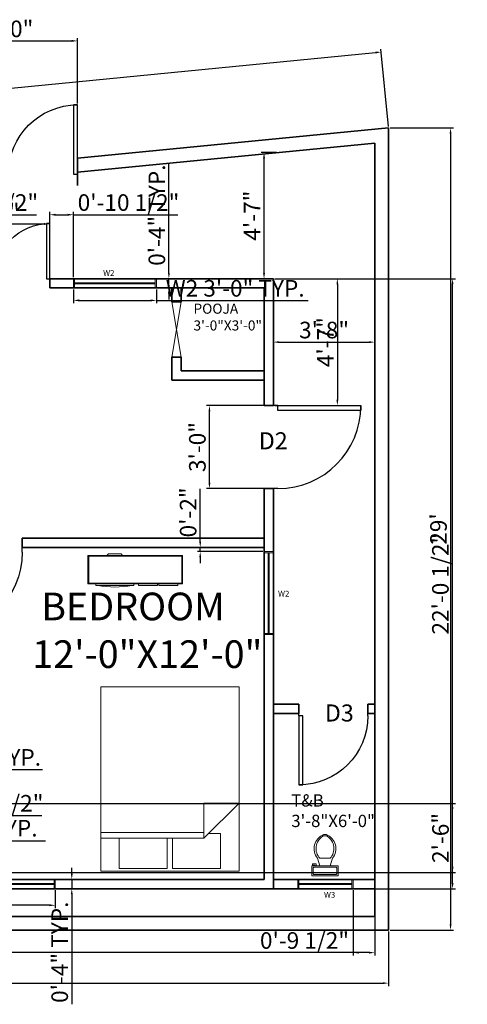
# Model space of a CAD drawing. Units: inches. Extents: x 2165 to 6441, y 2023 to 4425.
# Tile 3 of 4: x 2534 to 2728, y 2025 to 2452. Entities that reach past the tile are written whole.
import ezdxf

# ---------------------------------------------------------------- set-up
doc = ezdxf.new("R2010")
doc.units = ezdxf.units.IN
for name, color, linetype, lineweight in [('A-ANNO-DIMS', 7, 'Continuous', 18), ('A-ANNO-TEXT', 1, 'Continuous', 18), ('A-AREA-IDEN', 1, 'Continuous', 25), ('A-FLOR-FIXT', 9, 'Continuous', 18), ('C-PROP', 7, 'Continuous', 35), ('doors', 5, 'Continuous', 25), ('furniture', 9, 'Continuous', 18), ('walls', 7, 'Continuous', 35), ('windows', 72, 'Continuous', 18)]:
    doc.layers.add(name, color=color, linetype=linetype, lineweight=lineweight)
doc.styles.get("Standard").update_dxf_attribs({"font": 'arial.ttf'})
doc.dimstyles.new('ISO-25', dxfattribs={"dimtxt": 7.203125, "dimasz": 2.5, "dimexe": 1.25, "dimexo": 0.625, "dimtad": 1, "dimdec": 0, "dimlunit": 4, "dimtxsty": 'Standard', "dimcen": 2.5, "dimadec": 0, "dimazin": 0, "dimtfac": 1, "dimtdec": 0, "dimtmove": 0, "dimatfit": 3, "dimfxl": 1, "dimarcsym": 0})

# ---------------------------------------------------------------- blocks, each defined once
blk = doc.blocks.new('*U2')
for p, q in [((0, 0), (0, -5)), ((30, 0), (30, -5))]:
    blk.add_line(p, q)
blk.add_lwpolyline([(0, 0), (0, 30), (1.75, 30), (1.75, 0)], close=True)
blk.add_arc((0, 0), 30, 0, 90)
blk = doc.blocks.new('Bed - Queen')
for p, q in [((0, -80.00003), (0, 0)), ((0, 0), (59.99999, 0)), ((59.99999, 0), (59.99999, -80.00003)), ((7.99999, -1.2), (28.79998, -1.2)), ((7.99999, -14.4), (7.99999, -1.2)), ((28.79998, -1.2), (28.79998, -14.4)), ((31.19999, -1.2), (51.99999, -1.2)), ((31.19999, -14.4), (31.19999, -1.2)), ((51.99999, -1.2), (51.99999, -16.4)), ((0, -14.4), (44.8, -14.4)), ((44.8, -16.8), (0, -16.8)), ((59.99999, -29.6), (44.8, -14.4)), ((44.8, -14.4), (44.8, -29.6)), ((51.99999, -16.4), (46.79936, -16.4)), ((44.8, -29.6), (59.99999, -29.6)), ((59.99999, -80.00003), (0, -80.00003))]:
    blk.add_line(p, q)
blk = doc.blocks.new('Toilet - top')
for p, q in [((9.5, -6), (9.5, -2)), ((-10, -8.5), (-8, -8.5)), ((-10, -9.5), (-10, -8.5)), ((-7, -9.5), (-10, -9.5)), ((-8, -8.5), (-8, -8)), ((-7, -8), (-7, -9.5)), ((-4, -8), (-6, -14)), ((4, -14), (-4, -14)), ((4, -8), (6, -14))]:
    blk.add_line(p, q)
blk.add_lwpolyline([(10.5, -8), (10.5, 0), (-10.5, 0), (-10.5, -8)], close=True)
for points in [[(-9.5, -2), (-9.5, -6)], [(8.5, -1), (-8.5, -1)], [(-8.5, -7), (8.5, -7)]]:
    blk.add_lwpolyline(points)
for centre, radius, start, end in [((-8.62, -1.88), 0.884, 81.8699, 188.1301), ((-8.62, -6.12), 0.884, 171.8699, 278.1301), ((8.62, -1.88), 0.884, 351.8699, 98.1301), ((8.62, -6.12), 0.884, 261.8699, 8.1301), ((3.52, -21.58), 12.17, 141.46911, 247.97143), ((4.2, -21.82), 11.33, 136.36773, 238.94682), ((-3.52, -21.58), 12.17, 292.02843, 38.53071), ((-4.2, -21.82), 11.33, 301.05301, 43.63209), ((0, -27.88), 4, 245.73182, 294.26817), ((0, -29), 4, 254.86053, 285.13947)]:
    blk.add_arc(centre, radius, start, end)
blk = doc.blocks.new('*D8')
at = {"layer": 'A-ANNO-DIMS', "color": 0, "lineweight": -2, "transparency": 16777216}
for p, q in [((2693.62, 2405.41), (2690.35, 2438.92)), ((2200.96, 2389.92), (2687.99, 2437.43)), ((2201.62, 2357.41), (2198.35, 2390.92))]:
    blk.add_line(p, q, dxfattribs=at)
at = {"layer": 'A-ANNO-DIMS', "color": 0, "transparency": 16777216}
for points in [[(2687.95, 2437.85), (2688.03, 2437.02), (2690.48, 2437.67)], [(2200.92, 2390.33), (2201, 2389.5), (2198.48, 2389.67)]]:
    blk.add_solid(points, dxfattribs=at)
at = {"layer": 'Defpoints', "color": 0, "transparency": 16777216}
for p in [(2690.48, 2437.67), (2693.68, 2404.78), (2201.68, 2356.78)]:
    blk.add_point(p, dxfattribs=at)
at = {"layer": 'A-ANNO-DIMS', "color": 0, "transparency": 16777216, "insert": (2444.06, 2417.9), "char_height": 7.203, "attachment_point": 5, "rotation": 5.5722}
blk.add_mtext('41\'-2"', dxfattribs=at)
blk = doc.blocks.new('*D9')
at = {"layer": 'A-ANNO-DIMS', "color": 0, "lineweight": -2, "transparency": 16777216}
for p, q in [((2694.31, 2404.78), (2721.8, 2404.78)), ((2720.55, 2402.28), (2720.55, 2059.28)), ((2694.31, 2056.78), (2721.8, 2056.78))]:
    blk.add_line(p, q, dxfattribs=at)
at = {"layer": 'A-ANNO-DIMS', "color": 0, "transparency": 16777216}
for points in [[(2720.14, 2402.28), (2720.97, 2402.28), (2720.55, 2404.78)], [(2720.14, 2059.28), (2720.97, 2059.28), (2720.55, 2056.78)]]:
    blk.add_solid(points, dxfattribs=at)
at = {"layer": 'Defpoints', "color": 0, "transparency": 16777216}
for p in [(2693.68, 2404.78), (2693.68, 2056.78), (2720.55, 2056.78)]:
    blk.add_point(p, dxfattribs=at)
at = {"layer": 'A-ANNO-DIMS', "color": 0, "transparency": 16777216, "insert": (2716.25, 2230.78), "char_height": 7.203, "attachment_point": 5, "rotation": 90}
blk.add_mtext("29'", dxfattribs=at)
blk = doc.blocks.new('*D11')
at = {"layer": 'A-ANNO-DIMS', "color": 0, "lineweight": -2, "transparency": 16777216}
for p, q in [((2201.68, 2056.16), (2201.68, 2032.56)), ((2693.68, 2056.16), (2693.68, 2032.56)), ((2204.18, 2033.81), (2691.18, 2033.81))]:
    blk.add_line(p, q, dxfattribs=at)
at = {"layer": 'A-ANNO-DIMS', "color": 0, "transparency": 16777216}
for points in [[(2204.18, 2034.23), (2204.18, 2033.39), (2201.68, 2033.81)], [(2691.18, 2034.23), (2691.18, 2033.39), (2693.68, 2033.81)]]:
    blk.add_solid(points, dxfattribs=at)
at = {"layer": 'Defpoints', "color": 0, "transparency": 16777216}
for p in [(2201.68, 2056.78), (2693.68, 2056.78), (2693.68, 2033.81)]:
    blk.add_point(p, dxfattribs=at)
at = {"layer": 'A-ANNO-DIMS', "color": 0, "transparency": 16777216, "insert": (2447.68, 2038.05), "char_height": 7.203, "attachment_point": 5}
blk.add_mtext("41'", dxfattribs=at)
blk = doc.blocks.new('*D17')
at = {"layer": 'A-ANNO-DIMS', "color": 0, "lineweight": -2, "transparency": 16777216}
for p, q in [((2643.68, 2312.47), (2643.68, 2313.09)), ((2646.18, 2311.84), (2685.18, 2311.84)), ((2687.68, 2312.47), (2687.68, 2313.09))]:
    blk.add_line(p, q, dxfattribs=at)
at = {"layer": 'A-ANNO-DIMS', "color": 0, "transparency": 16777216}
for points in [[(2646.18, 2312.26), (2646.18, 2311.42), (2643.68, 2311.84)], [(2685.18, 2312.26), (2685.18, 2311.42), (2687.68, 2311.84)]]:
    blk.add_solid(points, dxfattribs=at)
at = {"layer": 'Defpoints', "color": 0, "transparency": 16777216}
for p in [(2643.68, 2311.84), (2687.68, 2311.84), (2687.68, 2311.84)]:
    blk.add_point(p, dxfattribs=at)
at = {"layer": 'A-ANNO-DIMS', "color": 0, "transparency": 16777216, "insert": (2665.68, 2316.15), "char_height": 7.203, "attachment_point": 5}
blk.add_mtext('3\'-8"', dxfattribs=at)
blk = doc.blocks.new('Entertainment Center')
for p, q in [((-4, 0), (-5, -1)), ((4, 0), (-4, 0)), ((5, -1), (4, 0)), ((-17, -19), (-17, -1)), ((-17, -1), (43, -1)), ((-16.5, -18.5), (-16.5, -1.5)), ((-16.5, -1.5), (42.5, -1.5)), ((42.5, -1.5), (42.5, -18.5)), ((43, -1), (43, -19)), ((42.5, -18.5), (-16.5, -18.5)), ((43, -19), (-17, -19)), ((-12, -20), (-12, -19)), ((12, -20), (-12, -20)), ((12, -19), (12, -20)), ((15, -20), (15, -19)), ((27, -20), (15, -20)), ((27, -19), (27, -20)), ((28, -20), (28, -19)), ((40, -20), (28, -20)), ((40, -19), (40, -20))]:
    blk.add_line(p, q)
blk.add_arc((0, 40), 61, 259.6111, 280.3889)
blk = doc.blocks.new('*D21')
at = {"layer": 'A-ANNO-DIMS', "color": 0, "lineweight": -2, "transparency": 16777216}
for p, q in [((2645.05, 2394.07), (2638.37, 2394.07)), ((2639.62, 2341.84), (2639.62, 2391.57)), ((2643.06, 2339.34), (2638.37, 2339.34))]:
    blk.add_line(p, q, dxfattribs=at)
at = {"layer": 'A-ANNO-DIMS', "color": 0, "transparency": 16777216}
for points in [[(2639.2, 2391.57), (2640.03, 2391.57), (2639.62, 2394.07)], [(2639.2, 2341.84), (2640.03, 2341.84), (2639.62, 2339.34)]]:
    blk.add_solid(points, dxfattribs=at)
at = {"layer": 'Defpoints', "color": 0, "transparency": 16777216}
for p in [(2639.62, 2394.07), (2645.67, 2394.07), (2643.68, 2339.34)]:
    blk.add_point(p, dxfattribs=at)
at = {"layer": 'A-ANNO-DIMS', "color": 0, "transparency": 16777216, "insert": (2635.39, 2366.71), "char_height": 7.203, "attachment_point": 5, "rotation": 90}
blk.add_mtext('4\'-7"', dxfattribs=at)
blk = doc.blocks.new('WIN-W2-36IN')
for p, q in [((0, 4), (36, 4)), ((0, 0), (0, 4)), ((36, 0), (0, 0)), ((0.5, 0), (0.5, 4)), ((0.5, 2.2), (35.5, 2.2)), ((0.5, 1.8), (35.5, 1.8)), ((0.5, 1.8), (35.5, 1.8)), ((35.5, 4), (35.5, 0)), ((36, 4), (36, 0))]:
    blk.add_line(p, q)
blk = doc.blocks.new('WIN-W1-48IN')
for p, q in [((0, 4), (48, 4)), ((0, 0), (0, 4)), ((48, 0), (0, 0)), ((0.5, 0), (0.5, 4)), ((0.5, 2.2), (47.5, 2.2)), ((0.5, 1.8), (47.5, 1.8)), ((47.5, 4), (47.5, 0)), ((48, 4), (48, 0))]:
    blk.add_line(p, q)
blk = doc.blocks.new('WIN-W3-24IN')
for p, q in [((0, 4), (24, 4)), ((0, 0), (0, 4)), ((24, 0), (0, 0)), ((0.5, 0), (0.5, 4)), ((23.5, 2.2), (0.5, 2.2)), ((23.5, 1.8), (0.5, 1.8)), ((23.5, 0), (23.5, 4)), ((24, 0), (24, 4))]:
    blk.add_line(p, q)
blk = doc.blocks.new('*D26')
at = {"layer": 'A-ANNO-DIMS', "color": 0, "lineweight": -2, "transparency": 16777216}
for p, q in [((2500.99, 2074.16), (2500.99, 2066.33)), ((2549, 2074.16), (2549, 2066.33)), ((2500.99, 2067.58), (2435.15, 2067.58)), ((2546.5, 2067.58), (2503.49, 2067.58))]:
    blk.add_line(p, q, dxfattribs=at)
at = {"layer": 'A-ANNO-DIMS', "color": 0, "transparency": 16777216}
for points in [[(2503.49, 2068), (2503.49, 2067.17), (2500.99, 2067.58)], [(2546.5, 2068), (2546.5, 2067.17), (2549, 2067.58)]]:
    blk.add_solid(points, dxfattribs=at)
at = {"layer": 'Defpoints', "color": 0, "transparency": 16777216}
for p in [(2500.99, 2074.78), (2549, 2074.78), (2500.99, 2067.58)]:
    blk.add_point(p, dxfattribs=at)
at = {"layer": 'A-ANNO-DIMS', "color": 0, "transparency": 16777216, "insert": (2466.82, 2071.89), "char_height": 7.2031, "attachment_point": 5}
blk.add_mtext('W1 4\'-0" TYP.', dxfattribs=at)
blk = doc.blocks.new('*D27')
at = {"layer": 'A-ANNO-DIMS', "color": 0, "lineweight": -2, "transparency": 16777216}
for p, q in [((2556.2, 2081.28), (2556.2, 2083.78)), ((2549.62, 2078.78), (2557.45, 2078.78)), ((2556.2, 2078.78), (2556.2, 2074.78)), ((2549.62, 2074.78), (2557.45, 2074.78)), ((2556.2, 2072.28), (2556.2, 2024.63))]:
    blk.add_line(p, q, dxfattribs=at)
at = {"layer": 'A-ANNO-DIMS', "color": 0, "transparency": 16777216}
for points in [[(2555.78, 2081.28), (2556.61, 2081.28), (2556.2, 2078.78)], [(2555.78, 2072.28), (2556.61, 2072.28), (2556.2, 2074.78)]]:
    blk.add_solid(points, dxfattribs=at)
at = {"layer": 'Defpoints', "color": 0, "transparency": 16777216}
for p in [(2549, 2078.78), (2549, 2074.78), (2556.2, 2074.78)]:
    blk.add_point(p, dxfattribs=at)
at = {"layer": 'A-ANNO-DIMS', "color": 0, "transparency": 16777216, "insert": (2551.89, 2047.21), "char_height": 7.203, "attachment_point": 5, "rotation": 90}
blk.add_mtext('0\'-4" TYP.', dxfattribs=at)
blk = doc.blocks.new('*D28')
at = {"layer": 'A-ANNO-DIMS', "color": 0, "lineweight": -2, "transparency": 16777216}
for p, q in [((2556.93, 2334.72), (2556.93, 2328.69)), ((2592.94, 2334.72), (2592.94, 2328.69)), ((2559.43, 2329.94), (2590.44, 2329.94)), ((2592.94, 2329.94), (2658.78, 2329.94))]:
    blk.add_line(p, q, dxfattribs=at)
at = {"layer": 'A-ANNO-DIMS', "color": 0, "transparency": 16777216}
for points in [[(2559.43, 2330.36), (2559.43, 2329.52), (2556.93, 2329.94)], [(2590.44, 2330.36), (2590.44, 2329.52), (2592.94, 2329.94)]]:
    blk.add_solid(points, dxfattribs=at)
at = {"layer": 'Defpoints', "color": 0, "transparency": 16777216}
for p in [(2556.93, 2335.34), (2592.94, 2335.34), (2592.94, 2329.94)]:
    blk.add_point(p, dxfattribs=at)
at = {"layer": 'A-ANNO-DIMS', "color": 0, "transparency": 16777216, "insert": (2627.11, 2334.25), "char_height": 7.2031, "attachment_point": 5}
blk.add_mtext('W2 3\'-0" TYP.', dxfattribs=at)
blk = doc.blocks.new('*D29')
at = {"layer": 'A-ANNO-DIMS', "color": 0, "lineweight": -2, "transparency": 16777216}
for p, q in [((2598.34, 2341.84), (2598.34, 2389.5)), ((2593.56, 2339.34), (2599.59, 2339.34)), ((2598.34, 2335.34), (2598.34, 2339.34)), ((2593.56, 2335.34), (2599.59, 2335.34)), ((2598.34, 2332.84), (2598.34, 2330.34))]:
    blk.add_line(p, q, dxfattribs=at)
at = {"layer": 'A-ANNO-DIMS', "color": 0, "transparency": 16777216}
for points in [[(2597.92, 2341.84), (2598.76, 2341.84), (2598.34, 2339.34)], [(2597.92, 2332.84), (2598.76, 2332.84), (2598.34, 2335.34)]]:
    blk.add_solid(points, dxfattribs=at)
at = {"layer": 'Defpoints', "color": 0, "transparency": 16777216}
for p in [(2592.94, 2339.34), (2598.34, 2339.34), (2592.94, 2335.34)]:
    blk.add_point(p, dxfattribs=at)
at = {"layer": 'A-ANNO-DIMS', "color": 0, "transparency": 16777216, "insert": (2594.04, 2366.92), "char_height": 7.203, "attachment_point": 5, "rotation": 90}
blk.add_mtext('0\'-4" TYP.', dxfattribs=at)
blk = doc.blocks.new('*D32')
at = {"layer": 'A-ANNO-DIMS', "color": 0, "lineweight": -2, "transparency": 16777216}
for p, q in [((2355.04, 2106.91), (2355.04, 2094.28)), ((2435.04, 2106.91), (2435.04, 2094.28)), ((2357.54, 2095.53), (2432.54, 2095.53)), ((2435.04, 2095.53), (2544.75, 2095.53))]:
    blk.add_line(p, q, dxfattribs=at)
at = {"layer": 'A-ANNO-DIMS', "color": 0, "transparency": 16777216}
for points in [[(2357.54, 2095.95), (2357.54, 2095.11), (2355.04, 2095.53)], [(2432.54, 2095.95), (2432.54, 2095.11), (2435.04, 2095.53)]]:
    blk.add_solid(points, dxfattribs=at)
at = {"layer": 'Defpoints', "color": 0, "transparency": 16777216}
for p in [(2355.04, 2107.53), (2435.04, 2107.53), (2435.04, 2095.53)]:
    blk.add_point(p, dxfattribs=at)
at = {"layer": 'A-ANNO-DIMS', "color": 0, "transparency": 16777216, "insert": (2491.14, 2100.1), "char_height": 7.2031, "attachment_point": 5}
blk.add_mtext('QUEEN BED 6\'-8" TYP.', dxfattribs=at)
blk = doc.blocks.new('*D43')
at = {"layer": 'A-ANNO-DIMS', "color": 0, "lineweight": -2, "transparency": 16777216}
for p, q in [((2461.96, 2128.52), (2461.96, 2125.2)), ((2473.4, 2128.52), (2473.4, 2125.2)), ((2464.46, 2126.45), (2470.9, 2126.45)), ((2473.4, 2126.45), (2543.44, 2126.45))]:
    blk.add_line(p, q, dxfattribs=at)
at = {"layer": 'A-ANNO-DIMS', "color": 0, "transparency": 16777216}
for points in [[(2464.46, 2126.86), (2464.46, 2126.03), (2461.96, 2126.45)], [(2470.9, 2126.86), (2470.9, 2126.03), (2473.4, 2126.45)]]:
    blk.add_solid(points, dxfattribs=at)
at = {"layer": 'Defpoints', "color": 0, "transparency": 16777216}
for p in [(2461.96, 2129.15), (2473.4, 2129.15), (2473.4, 2126.45)]:
    blk.add_point(p, dxfattribs=at)
at = {"layer": 'A-ANNO-DIMS', "color": 0, "transparency": 16777216, "insert": (2509.67, 2130.8), "char_height": 7.2031, "attachment_point": 5}
blk.add_mtext('0\'-11 1/2" TYP.', dxfattribs=at)
blk = doc.blocks.new('*D45')
at = {"layer": 'A-ANNO-DIMS', "color": 0, "lineweight": -2, "transparency": 16777216}
for p, q in [((2498.68, 2415.36), (2498.68, 2443.73)), ((2558.68, 2415.36), (2558.68, 2443.73)), ((2501.18, 2442.48), (2556.18, 2442.48))]:
    blk.add_line(p, q, dxfattribs=at)
at = {"layer": 'A-ANNO-DIMS', "color": 0, "transparency": 16777216}
for points in [[(2501.18, 2442.9), (2501.18, 2442.06), (2498.68, 2442.48)], [(2556.18, 2442.9), (2556.18, 2442.06), (2558.68, 2442.48)]]:
    blk.add_solid(points, dxfattribs=at)
at = {"layer": 'Defpoints', "color": 0, "transparency": 16777216}
for p in [(2558.68, 2442.48), (2498.68, 2414.73), (2558.68, 2414.73)]:
    blk.add_point(p, dxfattribs=at)
at = {"layer": 'A-ANNO-DIMS', "color": 0, "transparency": 16777216, "insert": (2528.68, 2446.78), "char_height": 7.203, "attachment_point": 5}
blk.add_mtext('5\'-0"', dxfattribs=at)
blk = doc.blocks.new('*D46')
at = {"layer": 'A-ANNO-DIMS', "color": 0, "lineweight": -2, "transparency": 16777216}
for p, q in [((2498.68, 2335.97), (2498.68, 2364.34)), ((2501.18, 2363.09), (2544.18, 2363.09)), ((2546.68, 2335.97), (2546.68, 2364.34))]:
    blk.add_line(p, q, dxfattribs=at)
at = {"layer": 'A-ANNO-DIMS', "color": 0, "transparency": 16777216}
for points in [[(2501.18, 2363.51), (2501.18, 2362.67), (2498.68, 2363.09)], [(2544.18, 2363.51), (2544.18, 2362.67), (2546.68, 2363.09)]]:
    blk.add_solid(points, dxfattribs=at)
at = {"layer": 'Defpoints', "color": 0, "transparency": 16777216}
for p in [(2546.68, 2363.09), (2498.68, 2335.34), (2546.68, 2335.34)]:
    blk.add_point(p, dxfattribs=at)
at = {"layer": 'A-ANNO-DIMS', "color": 0, "transparency": 16777216, "insert": (2522.68, 2367.39), "char_height": 7.203, "attachment_point": 5}
blk.add_mtext('4\'-0"', dxfattribs=at)
blk = doc.blocks.new('*D47')
at = {"layer": 'A-ANNO-DIMS', "color": 0, "lineweight": -2, "transparency": 16777216}
for p, q in [((2643.06, 2284.34), (2614.68, 2284.34)), ((2615.93, 2250.84), (2615.93, 2281.84)), ((2643.06, 2248.34), (2614.68, 2248.34))]:
    blk.add_line(p, q, dxfattribs=at)
at = {"layer": 'A-ANNO-DIMS', "color": 0, "transparency": 16777216}
for points in [[(2615.52, 2281.84), (2616.35, 2281.84), (2615.93, 2284.34)], [(2615.52, 2250.84), (2616.35, 2250.84), (2615.93, 2248.34)]]:
    blk.add_solid(points, dxfattribs=at)
at = {"layer": 'Defpoints', "color": 0, "transparency": 16777216}
for p in [(2615.93, 2284.34), (2643.68, 2284.34), (2643.68, 2248.34)]:
    blk.add_point(p, dxfattribs=at)
at = {"layer": 'A-ANNO-DIMS', "color": 0, "transparency": 16777216, "insert": (2611.63, 2266.34), "char_height": 7.203, "attachment_point": 5, "rotation": 90}
blk.add_mtext('3\'-0"', dxfattribs=at)
blk = doc.blocks.new('*D48')
at = {"layer": 'A-ANNO-DIMS', "color": 0, "lineweight": -2, "transparency": 16777216}
for p, q in [((2492.31, 2111.78), (2722.68, 2111.78)), ((2721.43, 2084.28), (2721.43, 2109.28)), ((2492.31, 2081.78), (2722.68, 2081.78))]:
    blk.add_line(p, q, dxfattribs=at)
at = {"layer": 'A-ANNO-DIMS', "color": 0, "transparency": 16777216}
for points in [[(2721.02, 2109.28), (2721.85, 2109.28), (2721.43, 2111.78)], [(2721.02, 2084.28), (2721.85, 2084.28), (2721.43, 2081.78)]]:
    blk.add_solid(points, dxfattribs=at)
at = {"layer": 'Defpoints', "color": 0, "transparency": 16777216}
for p in [(2491.68, 2111.78), (2721.43, 2111.78), (2491.68, 2081.78)]:
    blk.add_point(p, dxfattribs=at)
at = {"layer": 'A-ANNO-DIMS', "color": 0, "transparency": 16777216, "insert": (2717.13, 2096.78), "char_height": 7.203, "attachment_point": 5, "rotation": 90}
blk.add_mtext('2\'-6"', dxfattribs=at)
blk = doc.blocks.new('*D51')
at = {"layer": 'A-ANNO-DIMS', "color": 0, "lineweight": -2, "transparency": 16777216}
for p, q in [((2291.68, 2074.16), (2291.68, 2045.78)), ((2687.68, 2074.16), (2687.68, 2045.78)), ((2685.18, 2047.03), (2294.18, 2047.03))]:
    blk.add_line(p, q, dxfattribs=at)
at = {"layer": 'A-ANNO-DIMS', "color": 0, "transparency": 16777216}
for points in [[(2294.18, 2047.45), (2294.18, 2046.62), (2291.68, 2047.03)], [(2685.18, 2047.45), (2685.18, 2046.62), (2687.68, 2047.03)]]:
    blk.add_solid(points, dxfattribs=at)
at = {"layer": 'Defpoints', "color": 0, "transparency": 16777216}
for p in [(2291.68, 2074.78), (2687.68, 2074.78), (2291.68, 2047.03)]:
    blk.add_point(p, dxfattribs=at)
at = {"layer": 'A-ANNO-DIMS', "color": 0, "transparency": 16777216, "insert": (2489.68, 2051.34), "char_height": 7.203, "attachment_point": 5}
blk.add_mtext('33\'-0"', dxfattribs=at)
blk = doc.blocks.new('*D52')
at = {"layer": 'A-ANNO-DIMS', "color": 0, "lineweight": -2, "transparency": 16777216}
for p, q in [((2644.31, 2339.34), (2722.68, 2339.34)), ((2721.43, 2077.28), (2721.43, 2336.84)), ((2644.31, 2074.78), (2722.68, 2074.78))]:
    blk.add_line(p, q, dxfattribs=at)
at = {"layer": 'A-ANNO-DIMS', "color": 0, "transparency": 16777216}
for points in [[(2721.02, 2336.84), (2721.85, 2336.84), (2721.43, 2339.34)], [(2721.02, 2077.28), (2721.85, 2077.28), (2721.43, 2074.78)]]:
    blk.add_solid(points, dxfattribs=at)
at = {"layer": 'Defpoints', "color": 0, "transparency": 16777216}
for p in [(2643.68, 2339.34), (2721.43, 2339.34), (2643.68, 2074.78)]:
    blk.add_point(p, dxfattribs=at)
at = {"layer": 'A-ANNO-DIMS', "color": 0, "transparency": 16777216, "insert": (2717.08, 2207.06), "char_height": 7.203, "attachment_point": 5, "rotation": 90}
blk.add_mtext('22\'-0 1/2"', dxfattribs=at)
blk = doc.blocks.new('*D57')
at = {"layer": 'A-ANNO-DIMS', "color": 0, "lineweight": -2, "transparency": 16777216}
for p, q in [((2490.69, 2367.09), (2488.19, 2367.09)), ((2493.19, 2339.97), (2493.19, 2368.34)), ((2493.19, 2367.09), (2498.68, 2367.09)), ((2498.68, 2339.97), (2498.68, 2368.34)), ((2501.18, 2367.09), (2540.87, 2367.09))]:
    blk.add_line(p, q, dxfattribs=at)
at = {"layer": 'A-ANNO-DIMS', "color": 0, "transparency": 16777216}
for points in [[(2490.69, 2367.51), (2490.69, 2366.67), (2493.19, 2367.09)], [(2501.18, 2367.51), (2501.18, 2366.67), (2498.68, 2367.09)]]:
    blk.add_solid(points, dxfattribs=at)
at = {"layer": 'Defpoints', "color": 0, "transparency": 16777216}
for p in [(2498.68, 2367.09), (2493.19, 2339.34), (2498.68, 2339.34)]:
    blk.add_point(p, dxfattribs=at)
at = {"layer": 'A-ANNO-DIMS', "color": 0, "transparency": 16777216, "insert": (2522.28, 2371.44), "char_height": 7.203, "attachment_point": 5}
blk.add_mtext('0\'-5 1/2"', dxfattribs=at)
blk = doc.blocks.new('*D58')
at = {"layer": 'A-ANNO-DIMS', "color": 0, "lineweight": -2, "transparency": 16777216}
for p, q in [((2546.68, 2339.97), (2546.68, 2368.34)), ((2549.18, 2367.09), (2554.43, 2367.09)), ((2556.93, 2339.97), (2556.93, 2368.34)), ((2556.93, 2367.09), (2602.21, 2367.09))]:
    blk.add_line(p, q, dxfattribs=at)
at = {"layer": 'A-ANNO-DIMS', "color": 0, "transparency": 16777216}
for points in [[(2549.18, 2367.51), (2549.18, 2366.67), (2546.68, 2367.09)], [(2554.43, 2367.51), (2554.43, 2366.67), (2556.93, 2367.09)]]:
    blk.add_solid(points, dxfattribs=at)
at = {"layer": 'Defpoints', "color": 0, "transparency": 16777216}
for p in [(2556.93, 2367.09), (2546.68, 2339.34), (2556.93, 2339.34)]:
    blk.add_point(p, dxfattribs=at)
at = {"layer": 'A-ANNO-DIMS', "color": 0, "transparency": 16777216, "insert": (2580.82, 2371.44), "char_height": 7.203, "attachment_point": 5}
blk.add_mtext('0\'-10 1/2"', dxfattribs=at)
blk = doc.blocks.new('*D60')
at = {"layer": 'A-ANNO-DIMS', "color": 0, "lineweight": -2, "transparency": 16777216}
for p, q in [((2493.18, 2106.53), (2490.68, 2106.53)), ((2495.68, 2079.41), (2495.68, 2107.78)), ((2495.68, 2106.53), (2500.99, 2106.53)), ((2500.99, 2079.41), (2500.99, 2107.78)), ((2503.49, 2106.53), (2543.17, 2106.53))]:
    blk.add_line(p, q, dxfattribs=at)
at = {"layer": 'A-ANNO-DIMS', "color": 0, "transparency": 16777216}
for points in [[(2493.18, 2106.95), (2493.18, 2106.12), (2495.68, 2106.53)], [(2503.49, 2106.95), (2503.49, 2106.12), (2500.99, 2106.53)]]:
    blk.add_solid(points, dxfattribs=at)
at = {"layer": 'Defpoints', "color": 0, "transparency": 16777216}
for p in [(2500.99, 2106.53), (2495.68, 2078.78), (2500.99, 2078.78)]:
    blk.add_point(p, dxfattribs=at)
at = {"layer": 'A-ANNO-DIMS', "color": 0, "transparency": 16777216, "insert": (2524.58, 2110.88), "char_height": 7.203, "attachment_point": 5}
blk.add_mtext('0\'-5 1/2"', dxfattribs=at)
blk = doc.blocks.new('*D61')
at = {"layer": 'A-ANNO-DIMS', "color": 0, "lineweight": -2, "transparency": 16777216}
for p, q in [((2678.28, 2074.16), (2678.28, 2045.78)), ((2687.68, 2074.16), (2687.68, 2045.78)), ((2678.28, 2047.03), (2638.59, 2047.03)), ((2685.18, 2047.03), (2680.78, 2047.03))]:
    blk.add_line(p, q, dxfattribs=at)
at = {"layer": 'A-ANNO-DIMS', "color": 0, "transparency": 16777216}
for points in [[(2680.78, 2047.45), (2680.78, 2046.62), (2678.28, 2047.03)], [(2685.18, 2047.45), (2685.18, 2046.62), (2687.68, 2047.03)]]:
    blk.add_solid(points, dxfattribs=at)
at = {"layer": 'Defpoints', "color": 0, "transparency": 16777216}
for p in [(2678.28, 2074.78), (2687.68, 2074.78), (2678.28, 2047.03)]:
    blk.add_point(p, dxfattribs=at)
at = {"layer": 'A-ANNO-DIMS', "color": 0, "transparency": 16777216, "insert": (2657.18, 2051.38), "char_height": 7.203, "attachment_point": 5}
blk.add_mtext('0\'-9 1/2"', dxfattribs=at)
blk = doc.blocks.new('*D63')
at = {"layer": 'A-ANNO-DIMS', "color": 0, "lineweight": -2, "transparency": 16777216}
for p, q in [((2611.93, 2225.28), (2611.93, 2248.18)), ((2639.06, 2222.78), (2610.68, 2222.78)), ((2639.06, 2220.97), (2610.68, 2220.97)), ((2611.93, 2220.97), (2611.93, 2222.78)), ((2611.93, 2218.47), (2611.93, 2215.97))]:
    blk.add_line(p, q, dxfattribs=at)
at = {"layer": 'A-ANNO-DIMS', "color": 0, "transparency": 16777216}
for points in [[(2611.52, 2225.28), (2612.35, 2225.28), (2611.93, 2222.78)], [(2611.52, 2218.47), (2612.35, 2218.47), (2611.93, 2220.97)]]:
    blk.add_solid(points, dxfattribs=at)
at = {"layer": 'Defpoints', "color": 0, "transparency": 16777216}
for p in [(2611.93, 2222.78), (2639.68, 2222.78), (2639.68, 2220.97)]:
    blk.add_point(p, dxfattribs=at)
at = {"layer": 'A-ANNO-DIMS', "color": 0, "transparency": 16777216, "insert": (2607.63, 2237.98), "char_height": 7.203, "attachment_point": 5, "rotation": 90}
blk.add_mtext('0\'-2"', dxfattribs=at)
blk = doc.blocks.new('*D64')
at = {"layer": 'A-ANNO-DIMS', "color": 0, "lineweight": -2, "transparency": 16777216}
for p, q in [((2644.31, 2339.34), (2672.68, 2339.34)), ((2671.43, 2336.84), (2671.43, 2286.84)), ((2644.31, 2284.34), (2672.68, 2284.34))]:
    blk.add_line(p, q, dxfattribs=at)
at = {"layer": 'A-ANNO-DIMS', "color": 0, "transparency": 16777216}
for points in [[(2671.02, 2336.84), (2671.85, 2336.84), (2671.43, 2339.34)], [(2671.02, 2286.84), (2671.85, 2286.84), (2671.43, 2284.34)]]:
    blk.add_solid(points, dxfattribs=at)
at = {"layer": 'Defpoints', "color": 0, "transparency": 16777216}
for p in [(2643.68, 2339.34), (2643.68, 2284.34), (2671.43, 2284.34)]:
    blk.add_point(p, dxfattribs=at)
at = {"layer": 'A-ANNO-DIMS', "color": 0, "transparency": 16777216, "insert": (2667.21, 2311.84), "char_height": 7.203, "attachment_point": 5, "rotation": 90}
blk.add_mtext('4\'-7"', dxfattribs=at)

msp = doc.modelspace()

# ---------------------------------------------------------------- linework, layer by layer
at = {"layer": 'C-PROP'}
for p, q in [((2558.69, 2391.61), (2693.68, 2404.78)), ((2693.68, 2056.78), (2693.68, 2404.78)), ((2558.68, 2385.58), (2687.68, 2398.17)), ((2687.68, 2062.78), (2687.68, 2398.17)), ((2558.68, 2385.58), (2558.69, 2391.61)), ((2558.68, 2379.73), (2558.68, 2385.76)), ((2207.68, 2062.78), (2687.68, 2062.78)), ((2201.68, 2056.78), (2693.68, 2056.78))]:
    msp.add_line(p, q, dxfattribs=at)
at = {"layer": 'walls'}
for p, q in [((2643.68, 2339.34), (2546.68, 2339.34)), ((2546.68, 2339.34), (2546.68, 2335.34)), ((2643.68, 2284.34), (2643.68, 2339.34)), ((2639.68, 2335.34), (2546.68, 2335.34)), ((2599.68, 2329.34), (2599.68, 2335.34)), ((2603.68, 2335.34), (2603.68, 2329.34)), ((2603.68, 2329.34), (2603.68, 2335.34)), ((2639.68, 2284.34), (2639.68, 2335.34)), ((2603.68, 2329.34), (2599.68, 2329.34)), ((2599.68, 2295.34), (2599.68, 2305.34)), ((2599.68, 2305.34), (2603.68, 2305.34)), ((2603.68, 2299.34), (2603.68, 2305.34)), ((2639.68, 2299.34), (2603.68, 2299.34)), ((2639.68, 2295.34), (2599.68, 2295.34)), ((2639.68, 2284.34), (2643.68, 2284.34)), ((2639.68, 2284.34), (2643.68, 2284.34)), ((2639.68, 2078.78), (2639.68, 2248.34)), ((2643.68, 2248.34), (2639.68, 2248.34)), ((2643.68, 2074.78), (2643.68, 2248.34)), ((2534.68, 2226.78), (2534.68, 2222.78)), ((2534.68, 2226.78), (2639.68, 2226.78)), ((2534.68, 2222.78), (2639.68, 2222.78)), ((2643.68, 2154.78), (2654.68, 2154.78)), ((2654.68, 2154.78), (2654.68, 2150.78)), ((2684.68, 2150.78), (2684.68, 2154.78)), ((2684.68, 2154.78), (2687.68, 2154.78)), ((2643.68, 2150.78), (2654.68, 2150.78)), ((2687.68, 2150.78), (2684.68, 2150.78)), ((2684.68, 2150.78), (2687.68, 2150.78)), ((2443.68, 2078.78), (2639.68, 2078.78)), ((2643.68, 2078.78), (2687.68, 2078.78)), ((2291.68, 2074.78), (2643.68, 2074.78)), ((2643.68, 2074.78), (2687.68, 2074.78))]:
    msp.add_line(p, q, dxfattribs=at)
at = {"layer": 'windows'}
for p, q in [((2603.68, 2329.34), (2599.68, 2305.34)), ((2603.68, 2305.34), (2599.68, 2329.34))]:
    msp.add_line(p, q, dxfattribs=at)

# ---------------------------------------------------------------- block references
at = {"layer": 'A-FLOR-FIXT', "xscale": -0.5447974159761269, "yscale": 0.5447974159761269, "zscale": 0.5447974159761269, "rotation": 180}
msp.add_blockref('Toilet - top', (2666.07, 2080.33), dxfattribs=at)
at = {"layer": 'doors', "xscale": -1}
msp.add_blockref('*U2', (2558.68, 2384.73), dxfattribs=at)
at = {"layer": 'doors', "xscale": -0.8, "yscale": 0.8, "zscale": 0.8}
msp.add_blockref('*U2', (2546.68, 2339.34), dxfattribs=at)
at = {"layer": 'doors', "yscale": 1.199999999999999, "zscale": 1.199999999999999}
for p, xscale, rotation in [((2645.68, 2284.34), 1.199999999999999, 270), ((2498.68, 2220.78), -1.199999999999999, 180)]:
    msp.add_blockref('*U2', p, dxfattribs=dict(at, xscale=xscale, rotation=rotation))
at = {"layer": 'doors', "xscale": -1, "rotation": 180}
msp.add_blockref('*U2', (2654.68, 2149.78), dxfattribs=at)
at = {"layer": 'furniture', "xscale": 0.6851601597031488, "yscale": 0.6851601597031488, "zscale": 0.6851601597031488}
msp.add_blockref('Entertainment Center', (2574.85, 2220.01), dxfattribs=at)
at = {"layer": 'furniture', "xscale": -1, "rotation": 180}
msp.add_blockref('Bed - Queen', (2568.76, 2082.32), dxfattribs=at)
at = {"layer": 'windows'}
msp.add_blockref('WIN-W2-36IN', (2556.93, 2335.34), dxfattribs=at)
for name, p, rotation in [('WIN-W2-36IN', (2639.68, 2220.97), 269.9999999999984), ('WIN-W1-48IN', (2549, 2078.78), 180), ('WIN-W3-24IN', (2678.27, 2078.78), 180)]:
    msp.add_blockref(name, p, dxfattribs=dict(at, rotation=rotation))

# ---------------------------------------------------------------- texts
at = {"layer": 'A-ANNO-TEXT', "attachment_point": 1}
for s, width, gutter_width, heights, insert, char_height in [('W2', 0.1172, 12.5, [0], (2569.83, 2343.08), 2.5), ('D2', 3.6504, 37, [0], (2637.34, 2272.74), 7.4), ('W2', 0.1172, 12.5, [0], (2645.71, 2203.99), 2.5), ('D3', 7.3996, 37, [7.56], (2666.02, 2154.69), 7.4), ('W3', 0.1172, 12.5, [0], (2665.64, 2073.35), 2.5)]:
    msp.add_mtext_dynamic_manual_height_columns(s, width=width, gutter_width=gutter_width, heights=heights, dxfattribs=dict(at, insert=insert, char_height=char_height))
at = {"layer": 'A-AREA-IDEN', "attachment_point": 1}
for s, width, gutter_width, insert, char_height in [('POOJA\\P3\'-0"X3\'-0"', 1.254, 21.83, (2609, 2328.53), 4.3661), ('12\'-0"X12\'-0"', 0.3422, 12.5, (2539.05, 2182.5), 12), ('T&B\\P3\'-8"X6\'-0"', 5.3308, 26.65, (2651.45, 2115.72), 5.3308)]:
    msp.add_mtext_dynamic_manual_height_columns(s, width=width, gutter_width=gutter_width, heights=[0], dxfattribs=dict(at, insert=insert, char_height=char_height))
at = {"layer": 'A-AREA-IDEN', "insert": (2542.94, 2203.18), "char_height": 12, "attachment_point": 1, "rotation": 0.0167}
msp.add_mtext_dynamic_manual_height_columns('BEDROOM', width=1.7086, gutter_width=12.5, heights=[0], dxfattribs=at)

# ---------------------------------------------------------------- dimensions: what is measured, and where the dimension line sits
at = {"layer": 'A-ANNO-DIMS'}
for base, p1, p2, override, picture, middle in [((2558.68, 2442.48), (2498.68, 2414.73), (2558.68, 2414.73), {"dimdec": 1, "dimlfac": 1, "dimrnd": 0, "dimzin": 1, "dimdsep": 46, "dimlunit": 4, "dimfrac": 2}, '*D45', (2528.68, 2446.78)), ((2498.68, 2367.09), (2493.19, 2339.34), (2498.68, 2339.34), {"dimdec": 1, "dimlfac": 1, "dimrnd": 0, "dimzin": 1, "dimdsep": 46, "dimlunit": 4, "dimfrac": 2}, '*D57', (2522.28, 2371.44)), ((2556.9349, 2367.091), (2546.684, 2339.341), (2556.9349, 2339.341), {"dimdec": 1, "dimlfac": 1, "dimrnd": 0, "dimzin": 1, "dimdsep": 46, "dimlunit": 4, "dimfrac": 2}, '*D58', (2580.8242, 2371.4404)), ((2546.68, 2363.09), (2498.68, 2335.34), (2546.68, 2335.34), {"dimdec": 1, "dimlfac": 1, "dimrnd": 0, "dimzin": 1, "dimdsep": 46, "dimlunit": 4, "dimfrac": 2}, '*D46', (2522.68, 2367.39)), ((2687.68, 2311.84), (2643.68, 2311.84), (2687.68, 2311.84), {"dimclrd": 0, "dimclre": 0, "dimclrt": 0}, '*D17', (2665.68, 2316.15)), ((2693.68, 2033.81), (2201.68, 2056.78), (2693.68, 2056.78), {"dimclrd": 0, "dimclre": 0, "dimclrt": 0}, '*D11', (2447.68, 2038.05))]:
    dim = msp.add_linear_dim(base=base, p1=p1, p2=p2, dimstyle='ISO-25', override=override, dxfattribs=at)
    dim.commit()
    dim.dimension.update_dxf_attribs({"geometry": picture, "text_midpoint": middle})
dim = msp.add_aligned_dim(p1=(2201.68, 2356.78), p2=(2693.68, 2404.78), distance=33.05, dimstyle='ISO-25', override={"dimclrd": 0, "dimclre": 0, "dimclrt": 0}, dxfattribs=at)
dim.commit()
dim.dimension.update_dxf_attribs({"geometry": '*D8', "text_midpoint": (2444.06, 2417.9)})
for base, p1, p2, angle, override, picture, middle in [((2720.55, 2056.78), (2693.68, 2404.78), (2693.68, 2056.78), 90, {"dimclrd": 0, "dimclre": 0, "dimclrt": 0}, '*D9', (2716.25, 2230.78)), ((2639.62, 2394.07), (2643.68, 2339.34), (2645.67, 2394.07), 90, {"dimclrd": 0, "dimclre": 0, "dimclrt": 0}, '*D21', (2635.39, 2366.71)), ((2721.43, 2339.34), (2643.68, 2074.78), (2643.68, 2339.34), 90, {"dimdec": 1, "dimlfac": 1, "dimrnd": 0, "dimzin": 1, "dimdsep": 46, "dimlunit": 4, "dimfrac": 2}, '*D52', (2717.08, 2207.06)), ((2671.43, 2284.34), (2643.68, 2339.34), (2643.68, 2284.34), 270, {"dimdec": 1, "dimlfac": 1, "dimrnd": 0, "dimzin": 1, "dimdsep": 46, "dimlunit": 4, "dimfrac": 2}, '*D64', (2667.21, 2311.84)), ((2615.93, 2284.34), (2643.68, 2248.34), (2643.68, 2284.34), 90, {"dimdec": 1, "dimlfac": 1, "dimrnd": 0, "dimzin": 1, "dimdsep": 46, "dimlunit": 4, "dimfrac": 2}, '*D47', (2611.63, 2266.34)), ((2611.93, 2222.78), (2639.68, 2220.97), (2639.68, 2222.78), 90, {"dimdec": 1, "dimlfac": 1, "dimrnd": 0, "dimzin": 1, "dimdsep": 46, "dimlunit": 4, "dimfrac": 2}, '*D63', (2607.63, 2237.98)), ((2500.99, 2106.53), (2495.68, 2078.78), (2500.99, 2078.78), 0, {"dimdec": 1, "dimlfac": 1, "dimrnd": 0, "dimzin": 1, "dimdsep": 46, "dimlunit": 4, "dimfrac": 2}, '*D60', (2524.58, 2110.88)), ((2721.43, 2111.78), (2491.68, 2081.78), (2491.68, 2111.78), 90, {"dimdec": 1, "dimlfac": 1, "dimrnd": 0, "dimzin": 1, "dimdsep": 46, "dimlunit": 4, "dimfrac": 2}, '*D48', (2717.13, 2096.78)), ((2291.68, 2047.03), (2687.68, 2074.78), (2291.68, 2074.78), 180, {"dimdec": 1, "dimlfac": 1, "dimrnd": 0, "dimzin": 1, "dimdsep": 46, "dimlunit": 4, "dimfrac": 2}, '*D51', (2489.68, 2051.34)), ((2678.28, 2047.03), (2687.68, 2074.78), (2678.28, 2074.78), 180, {"dimdec": 1, "dimlfac": 1, "dimrnd": 0, "dimzin": 1, "dimdsep": 46, "dimlunit": 4, "dimfrac": 2}, '*D61', (2657.18, 2051.38))]:
    dim = msp.add_linear_dim(base=base, p1=p1, p2=p2, angle=angle, dimstyle='ISO-25', override=override, dxfattribs=at)
    dim.commit()
    dim.dimension.update_dxf_attribs({"geometry": picture, "text_midpoint": middle})
for base, p1, p2, angle, text, picture, middle in [((2598.34, 2339.34), (2592.94, 2335.34), (2592.94, 2339.34), 90, '<> TYP.', '*D29', (2594.04, 2366.92)), ((2500.99, 2067.58), (2549, 2074.78), (2500.99, 2074.78), 180, 'W1 <> TYP.', '*D26', (2466.82, 2071.89)), ((2556.2, 2074.78), (2549, 2078.78), (2549, 2074.78), 270, '<> TYP.', '*D27', (2551.89, 2047.21))]:
    dim = msp.add_linear_dim(base=base, p1=p1, p2=p2, angle=angle, text=text, dimstyle='ISO-25', override={"dimdec": 1, "dimlfac": 1, "dimrnd": 0, "dimzin": 1, "dimdsep": 46, "dimlunit": 4, "dimfrac": 2}, dxfattribs=at)
    dim.commit()
    dim.dimension.update_dxf_attribs({"geometry": picture, "text_midpoint": middle})
for base, p1, p2, text, picture, middle in [((2592.94, 2329.94), (2556.93, 2335.34), (2592.94, 2335.34), 'W2 <> TYP.', '*D28', (2627.11, 2334.25)), ((2473.4, 2126.45), (2461.96, 2129.15), (2473.4, 2129.15), '<> TYP.', '*D43', (2509.67, 2130.8)), ((2435.04, 2095.53), (2355.04, 2107.53), (2435.04, 2107.53), 'QUEEN BED <> TYP.', '*D32', (2491.14, 2100.1))]:
    dim = msp.add_linear_dim(base=base, p1=p1, p2=p2, text=text, dimstyle='ISO-25', override={"dimdec": 1, "dimlfac": 1, "dimrnd": 0, "dimzin": 1, "dimdsep": 46, "dimlunit": 4, "dimfrac": 2}, dxfattribs=at)
    dim.commit()
    dim.dimension.update_dxf_attribs({"geometry": picture, "text_midpoint": middle})

doc.saveas('drawing.dxf')
